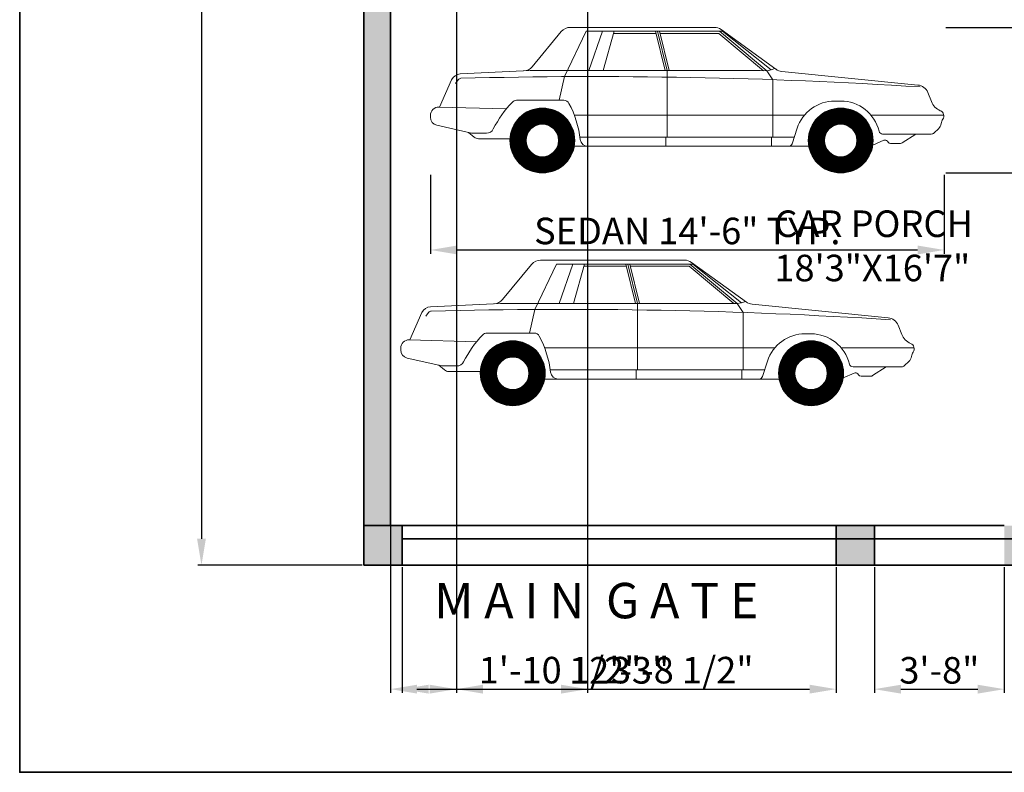
# Model space of a CAD drawing. Units: inches. Extents: x 32476 to 33108, y 58720 to 59630.
# Tile 1 of 6: x 32476 to 32810, y 58720 to 58975. Entities that reach past the tile are written whole.
import ezdxf

# ---------------------------------------------------------------- set-up
doc = ezdxf.new("R2010")
doc.units = ezdxf.units.IN
for name, color, linetype, lineweight in [('A-ANNO-DIMS', 6, 'Continuous', 18), ('A-ANNO-TEXT', 3, 'Continuous', 18), ('A-ANNO-TTLB', 7, 'Continuous', 35), ('A-AREA-IDEN', 32, 'Continuous', 18), ('A-EQPM-VEHI', 8, 'Continuous', 18), ('A-SITE-GATE', 7, 'Continuous', 35), ('A-SITE-PATT', 242, 'Continuous', 13), ('A-WALL', 7, 'Continuous', 35), ('A-WALL-PATT', 251, 'Continuous', 13)]:
    doc.layers.add(name, color=color, linetype=linetype, lineweight=lineweight)
doc.styles.get("Standard").update_dxf_attribs({"font": 'arial.ttf'})
doc.dimstyles.new('ISO-25', dxfattribs={"dimtxt": 9, "dimasz": 9, "dimexe": 1.25, "dimexo": 0.625, "dimtad": 1, "dimdec": 1, "dimrnd": 9, "dimlunit": 3, "dimtxsty": 'Standard', "dimcen": 2.5, "dimadec": 0, "dimazin": 0, "dimtfac": 1, "dimtdec": 1, "dimtmove": 0, "dimatfit": 3, "dimfxl": 1, "dimarcsym": 0})

# ---------------------------------------------------------------- blocks, each defined once
blk = doc.blocks.new('*D2')
at = {"layer": 'A-ANNO-DIMS', "color": 0, "lineweight": -2, "transparency": 16777216}
for p, q in [((32592.41, 59486.22), (32536.75, 59486.22)), ((32538, 59477.22), (32538, 58799.22)), ((32592.41, 58790.22), (32536.75, 58790.22))]:
    blk.add_line(p, q, dxfattribs=at)
at = {"layer": 'A-ANNO-DIMS', "color": 0, "transparency": 16777216}
for points in [[(32536.5, 59477.22), (32539.5, 59477.22), (32538, 59486.22)], [(32536.5, 58799.22), (32539.5, 58799.22), (32538, 58790.22)]]:
    blk.add_solid(points, dxfattribs=at)
at = {"layer": 'Defpoints', "color": 0, "transparency": 16777216}
for p in [(32593.04, 59486.22), (32538, 58790.22), (32593.04, 58790.22)]:
    blk.add_point(p, dxfattribs=at)
at = {"layer": 'A-ANNO-DIMS', "color": 0, "transparency": 16777216, "insert": (32532.78, 59138.22), "char_height": 9, "attachment_point": 5, "rotation": 90}
blk.add_mtext('57\'-9"', dxfattribs=at)
blk = doc.blocks.new('Car - sedan  side')
for p, q in [((-139.53, 35.99), (-129.64, 47.91)), ((-128.57, 32.64), (-121.22, 48.02)), ((-77.81, 49.34), (-126.58, 49.34)), ((-74.7, 48.02), (-121.22, 48.02)), ((-120.32, 34.67), (-115.67, 48.02)), ((-115.4, 34.67), (-111.74, 48.02)), ((-97.55, 47.3), (-111.94, 47.3)), ((-94.41, 34.67), (-97.73, 48.02)), ((-93.72, 34.67), (-97.04, 48.02)), ((-93.03, 34.67), (-96.34, 48.02)), ((-76.26, 47.3), (-96.16, 47.3)), ((-61.08, 34.66), (-76.26, 47.3)), ((-60.02, 34.65), (-76.07, 48.02)), ((-56.87, 35.13), (-75.48, 48.59)), ((-58.54, 34.93), (-74.99, 48.02)), ((-140.23, 34.67), (-163.88, 33.56)), ((-62.28, 34.67), (-140.23, 34.67)), ((-93.72, 19.62), (-93.72, 34.67)), ((-62.28, 34.67), (-60.02, 34.65)), ((-60.02, 34.65), (-58.54, 34.93)), ((-57.97, 31.61), (-60.02, 34.65)), ((-57.21, 35.38), (-58.54, 34.93)), ((-54.93, 34.4), (-8.75, 29.8)), ((-170.93, 22.32), (-166.81, 31.56)), ((-164.57, 31.6), (-165.48, 30.35)), ((-130.39, 24.63), (-128.57, 32.64)), ((-57.97, 19.62), (-57.97, 31.61)), ((-4.21, 24.18), (-5.42, 27.27)), ((-128.78, 24.63), (-144.79, 24.63)), ((-36.97, 24.38), (-34.94, 24.38)), ((-148.26, 21.7), (-171.11, 22.33)), ((-174, 19.51), (-174, 18.91)), ((-47.2, 19.62), (-125.23, 19.62)), ((-93.72, 12.14), (-93.72, 19.62)), ((-57.97, 12.14), (-57.97, 19.62)), ((0, 19.62), (-24.7, 19.62)), ((-160.12, 13.48), (-171.81, 16.16)), ((-159.22, 12.14), (-161.08, 13.7)), ((-155.01, 13.48), (-160.12, 13.48)), ((-51.4, 9.89), (-49.69, 15.14)), ((-3.22, 13.59), (-1.77, 14.97)), ((-147.03, 11.6), (-157.73, 11.6)), ((-50.67, 12.14), (-123.32, 12.14)), ((-94.21, 9.03), (-94.21, 12.14)), ((-58.39, 9.03), (-58.39, 12.14)), ((-20.36, 11.06), (-24.06, 9.44)), ((-4.23, 13.19), (-20.72, 13.19)), ((-18.83, 10.42), (-19.11, 10.76)), ((-14.68, 10.03), (-18.01, 10.03)), ((-9.5, 13.19), (-14.1, 10.2)), ((-120.62, 9.03), (-125.23, 9.03)), ((-45.76, 9.03), (-120.62, 9.03))]:
    blk.add_line(p, q)
at = {"const_width": 5.49}
for points in [[(-127.8, 11, -1), (-144.3, 11, -1)], [(-26.69, 11, -1), (-43.19, 11, -1)]]:
    blk.add_lwpolyline(points, format="xyb", close=True, dxfattribs=at)
for centre, radius in [((-136.05, 11), 11), ((-34.94, 11), 11), ((-136.05, 11), 5.51), ((-34.94, 11), 5.51)]:
    blk.add_circle(centre, radius)
for centre, radius, start, end in [((-126.58, 45.38), 3.97, 90, 140.3029), ((-77.81, 45.38), 3.97, 54.135, 90), ((-163.72, 30.18), 3.38, 92.6827, 155.9736), ((-142.58, 38.53), 3.97, 272.6827, 320.3029), ((-54.54, 38.35), 3.97, 234.135, 264.3123), ((-163.62, 30.91), 1.17, 91.491, 143.9553), ((-118.51, -1702.12), 1734.79, 86.34698, 91.49105), ((-9.15, 25.82), 4, 21.3107, 84.3123), ((-118.09, -2.78), 38.85, 136.3964, 152.9097), ((-144.79, 22.64), 1.98, 90, 136.3964), ((-128.78, 22.64), 1.98, 28.1371, 90), ((-157.14, 7.48), 34.14, 6.5135, 28.1371), ((-36.97, 11), 13.38, 90, 161.9732), ((-34.94, 11), 13.38, 13.5864, 90), ((0.9, 26.18), 5.49, 201.3107, 247.7048), ((-171.18, 19.51), 2.82, 88.4193, 180), ((-1.92, 19.3), 1.94, 325.3744, 67.7048), ((-171.18, 18.91), 2.82, 180, 257.0905), ((-3.82, 17.12), 2.96, 313.7173, 352.3839), ((2.46, 16.28), 3.37, 145.3744, 172.3839), ((-155.01, 16.1), 2.62, 270, 332.9097), ((-20.72, 14.43), 1.24, 193.5864, 270), ((-4.23, 14.65), 1.46, 270, 313.7173), ((-157.73, 13.93), 2.32, 230.1291, 270), ((-120.62, 11.65), 2.62, 186.5135, 270), ((-19.93, 10.09), 1.06, 39.301, 113.7159), ((-18.01, 11.09), 1.06, 219.301, 270), ((-14.68, 11.09), 1.06, 270, 303.047), ((-52.58, 10.27), 1.24, 270, 341.9732)]:
    blk.add_arc(centre, radius, start, end)
blk = doc.blocks.new('*D23')
at = {"layer": 'A-ANNO-DIMS', "color": 0, "lineweight": -2, "transparency": 16777216}
for p, q in [((32615.59, 58922.56), (32615.59, 58895.82)), ((32789.71, 58922.56), (32789.71, 58895.82)), ((32624.59, 58897.07), (32780.71, 58897.07))]:
    blk.add_line(p, q, dxfattribs=at)
at = {"layer": 'A-ANNO-DIMS', "color": 0, "transparency": 16777216}
for points in [[(32624.59, 58898.57), (32624.59, 58895.57), (32615.59, 58897.07)], [(32780.71, 58898.57), (32780.71, 58895.57), (32789.71, 58897.07)]]:
    blk.add_solid(points, dxfattribs=at)
at = {"layer": 'Defpoints', "color": 0, "transparency": 16777216}
for p in [(32615.59, 58923.18), (32789.71, 58923.18), (32789.71, 58897.07)]:
    blk.add_point(p, dxfattribs=at)
at = {"layer": 'A-ANNO-DIMS', "color": 0, "transparency": 16777216, "insert": (32702.65, 58902.35), "char_height": 9, "attachment_point": 5}
blk.add_mtext('SEDAN 14\'-6" TYP.', dxfattribs=at)
blk = doc.blocks.new('*D24')
at = {"layer": 'A-ANNO-DIMS', "color": 0, "lineweight": -2, "transparency": 16777216}
for p, q in [((32815.82, 58972.53), (32815.82, 59058.97)), ((32790.33, 58972.53), (32817.07, 58972.53)), ((32815.82, 58932.18), (32815.82, 58963.53)), ((32790.33, 58923.18), (32817.07, 58923.18))]:
    blk.add_line(p, q, dxfattribs=at)
at = {"layer": 'A-ANNO-DIMS', "color": 0, "transparency": 16777216}
for points in [[(32814.32, 58963.53), (32817.32, 58963.53), (32815.82, 58972.53)], [(32814.32, 58932.18), (32817.32, 58932.18), (32815.82, 58923.18)]]:
    blk.add_solid(points, dxfattribs=at)
at = {"layer": 'Defpoints', "color": 0, "transparency": 16777216}
for p in [(32789.71, 58972.53), (32815.82, 58972.53), (32789.71, 58923.18)]:
    blk.add_point(p, dxfattribs=at)
at = {"layer": 'A-ANNO-DIMS', "color": 0, "transparency": 16777216, "insert": (32810.54, 59020.25), "char_height": 9, "attachment_point": 5, "rotation": 90}
blk.add_mtext('4\'-1 1/2" TYP.', dxfattribs=at)
blk = doc.blocks.new('*D37')
at = {"layer": 'A-ANNO-DIMS', "color": 0, "lineweight": -2, "transparency": 16777216}
for p, q in [((32605.97, 58789.59), (32605.97, 58746.97)), ((32753.12, 58789.59), (32753.12, 58746.97)), ((32614.97, 58748.22), (32744.12, 58748.22))]:
    blk.add_line(p, q, dxfattribs=at)
at = {"layer": 'A-ANNO-DIMS', "color": 0, "transparency": 16777216}
for points in [[(32614.97, 58749.72), (32614.97, 58746.72), (32605.97, 58748.22)], [(32744.12, 58749.72), (32744.12, 58746.72), (32753.12, 58748.22)]]:
    blk.add_solid(points, dxfattribs=at)
at = {"layer": 'Defpoints', "color": 0, "transparency": 16777216}
for p in [(32605.97, 58790.22), (32753.12, 58790.22), (32753.12, 58748.22)]:
    blk.add_point(p, dxfattribs=at)
at = {"layer": 'A-ANNO-DIMS', "color": 0, "transparency": 16777216, "insert": (32679.55, 58753.44), "char_height": 9, "attachment_point": 5}
blk.add_mtext('12\'-3"', dxfattribs=at)
blk = doc.blocks.new('*D38')
at = {"layer": 'A-ANNO-DIMS', "color": 0, "lineweight": -2, "transparency": 16777216}
for p, q in [((32766.06, 58789.59), (32766.06, 58746.97)), ((32810.1, 58789.59), (32810.1, 58746.97)), ((32775.06, 58748.22), (32801.1, 58748.22))]:
    blk.add_line(p, q, dxfattribs=at)
at = {"layer": 'A-ANNO-DIMS', "color": 0, "transparency": 16777216}
for points in [[(32775.06, 58749.72), (32775.06, 58746.72), (32766.06, 58748.22)], [(32801.1, 58749.72), (32801.1, 58746.72), (32810.1, 58748.22)]]:
    blk.add_solid(points, dxfattribs=at)
at = {"layer": 'Defpoints', "color": 0, "transparency": 16777216}
for p in [(32766.06, 58790.22), (32810.1, 58790.22), (32810.1, 58748.22)]:
    blk.add_point(p, dxfattribs=at)
at = {"layer": 'A-ANNO-DIMS', "color": 0, "transparency": 16777216, "insert": (32788.08, 58753.44), "char_height": 9, "attachment_point": 5}
blk.add_mtext('3\'-8"', dxfattribs=at)
blk = doc.blocks.new('*D45')
at = {"layer": 'A-ANNO-DIMS', "color": 0, "lineweight": -2, "transparency": 16777216}
for p, q in [((32602.04, 59010.09), (32602.04, 58746.97)), ((32624.39, 59010.09), (32624.39, 58746.97)), ((32611.04, 58748.22), (32615.39, 58748.22)), ((32624.39, 58748.22), (32685.68, 58748.22))]:
    blk.add_line(p, q, dxfattribs=at)
at = {"layer": 'A-ANNO-DIMS', "color": 0, "transparency": 16777216}
for points in [[(32611.04, 58749.72), (32611.04, 58746.72), (32602.04, 58748.22)], [(32615.39, 58749.72), (32615.39, 58746.72), (32624.39, 58748.22)]]:
    blk.add_solid(points, dxfattribs=at)
at = {"layer": 'Defpoints', "color": 0, "transparency": 16777216}
for p in [(32602.04, 59010.72), (32624.39, 59010.72), (32624.39, 58748.22)]:
    blk.add_point(p, dxfattribs=at)
at = {"layer": 'A-ANNO-DIMS', "color": 0, "transparency": 16777216, "insert": (32659.53, 58753.5), "char_height": 9, "attachment_point": 5}
blk.add_mtext('1\'-10 1/2"', dxfattribs=at)
blk = doc.blocks.new('*D46')
at = {"layer": 'A-ANNO-DIMS', "color": 0, "lineweight": -2, "transparency": 16777216}
for p, q in [((32624.39, 59010.09), (32624.39, 58746.97)), ((32668.87, 59010.09), (32668.87, 58746.97)), ((32633.39, 58748.22), (32659.87, 58748.22)), ((32668.87, 58748.22), (32724.01, 58748.22))]:
    blk.add_line(p, q, dxfattribs=at)
at = {"layer": 'A-ANNO-DIMS', "color": 0, "transparency": 16777216}
for points in [[(32633.39, 58749.72), (32633.39, 58746.72), (32624.39, 58748.22)], [(32659.87, 58749.72), (32659.87, 58746.72), (32668.87, 58748.22)]]:
    blk.add_solid(points, dxfattribs=at)
at = {"layer": 'Defpoints', "color": 0, "transparency": 16777216}
for p in [(32624.39, 59010.72), (32668.87, 59010.72), (32668.87, 58748.22)]:
    blk.add_point(p, dxfattribs=at)
at = {"layer": 'A-ANNO-DIMS', "color": 0, "transparency": 16777216, "insert": (32700.94, 58753.5), "char_height": 9, "attachment_point": 5}
blk.add_mtext('3\'-8 1/2"', dxfattribs=at)

msp = doc.modelspace()

# ---------------------------------------------------------------- hatches: boundary and pattern name
at = {"layer": 'A-SITE-PATT'}
h = msp.add_hatch(color=256, dxfattribs=at)
h.dxf.hatch_style = 1
h.paths.add_polyline_path([(32605.97, 58803.66), (32593.04, 58803.66), (32593.04, 58790.22), (32605.97, 58790.22)])
h.paths.add_polyline_path([(32766.06, 58799.22), (32753.12, 58799.22), (32753.12, 58790.22), (32766.06, 58790.22)])
h.paths.add_polyline_path([(32766.06, 58803.66), (32753.12, 58803.66), (32753.12, 58799.22), (32766.06, 58799.22)])
h.paths.add_polyline_path([(32823.04, 58799.22), (32810.1, 58799.22), (32810.1, 58790.22), (32823.04, 58790.22)])
h.paths.add_polyline_path([(32823.04, 58803.66), (32810.1, 58803.66), (32810.1, 58799.22), (32823.04, 58799.22)])
at = {"layer": 'A-WALL-PATT'}
h = msp.add_hatch(color=256, dxfattribs=at)
h.dxf.hatch_style = 1
h.paths.add_polyline_path([(32602.04, 59418.72), (32606.39, 59418.72), (32606.39, 59423.22), (32602.04, 59423.22), (32602.04, 59477.22), (32698.04, 59477.22), (32698.04, 59469.73), (32702.54, 59469.73), (32702.54, 59481.72), (32867.54, 59481.72), (32867.54, 59427.72), (32860.2, 59427.72), (32860.2, 59418.72), (32867.54, 59418.72), (32935.14, 59418.72), (32935.14, 59423.22), (32872.04, 59423.22), (32872.04, 59477.22), (32968.04, 59477.22), (32968.04, 59423.22), (32962.36, 59423.22), (32962.36, 59418.72), (32968.04, 59418.72), (32968.04, 59286.72), (32867.54, 59286.72), (32832.04, 59286.72), (32828.7, 59289.44), (32818.99, 59279.82), (32823.04, 59277.72), (32823.04, 59269.52), (32832.04, 59269.52), (32832.04, 59277.72), (32867.54, 59277.72), (32968.04, 59277.72), (32968.04, 58880.22), (32925.88, 58880.22), (32925.88, 58871.22), (32968.04, 58871.22), (32968.04, 58799.22), (32823.04, 58799.22), (32823.04, 58790.22), (32977.04, 58790.22), (32977.04, 59486.22), (32867.54, 59486.22), (32702.54, 59486.22), (32593.04, 59486.22), (32593.04, 58803.66), (32602.04, 58803.66), (32602.04, 59001.72), (32624.39, 59001.72), (32624.39, 59010.72), (32602.04, 59010.72), (32602.04, 59124.72), (32648.65, 59124.72), (32648.65, 59133.72), (32602.04, 59133.72), (32602.04, 59277.72), (32757.41, 59277.72), (32757.41, 59279.22), (32742.07, 59288.84), (32739.6, 59286.72), (32702.54, 59286.72), (32602.04, 59286.72)])
h.paths.add_polyline_path([(32763.92, 59133.72), (32685.69, 59133.72), (32685.69, 59124.72), (32693.04, 59124.72), (32693.04, 59010.72), (32668.87, 59010.72), (32668.87, 59001.72), (32705.76, 59001.72), (32705.76, 59010.72), (32702.04, 59010.72), (32702.04, 59124.72), (32763.92, 59124.72)], flags=17)
h.paths.add_polyline_path([(32832.04, 59226.49), (32823.04, 59226.49), (32823.04, 59133.72), (32814.31, 59133.72), (32814.31, 59124.72), (32823.04, 59124.72), (32823.04, 59099.14), (32832.04, 59099.14), (32832.04, 59124.72), (32839.29, 59124.72), (32839.29, 59133.72), (32832.04, 59133.72)], flags=17)
h.paths.add_polyline_path([(32921.54, 59133.72), (32874.43, 59133.72), (32874.43, 59124.72), (32917.04, 59124.72), (32917.04, 59097.72), (32921.54, 59097.72), (32921.54, 59124.72)], flags=17)
h.paths.add_polyline_path([(32832.04, 59066.22), (32968.04, 59066.22), (32968.04, 59070.72), (32921.54, 59070.72), (32921.54, 59074.56), (32917.04, 59074.56), (32917.04, 59070.72), (32832.04, 59070.72), (32832.04, 59074.32), (32823.04, 59074.32), (32823.04, 59056.98), (32832.04, 59056.98)], flags=17)
h.paths.add_polyline_path([(32738.1, 59010.72), (32721.79, 59010.72), (32721.79, 59001.72), (32738.1, 59001.72)], flags=16)
h.paths.add_polyline_path([(32763.19, 59010.72), (32754.77, 59010.72), (32754.77, 59001.72), (32763.19, 59001.72)], flags=16)
h.paths.add_polyline_path([(32832.04, 59016.15), (32823.04, 59016.15), (32823.04, 59010.72), (32814.31, 59010.72), (32814.31, 59001.72), (32823.04, 59001.72), (32823.04, 58871.22), (32860.05, 58871.22), (32860.05, 58880.22), (32832.04, 58880.22)], flags=17)
h.paths.add_polyline_path([(32702.54, 59448.33), (32698.04, 59448.33), (32698.04, 59423.22), (32631.9, 59423.22), (32631.9, 59418.72), (32702.54, 59418.72), (32706.18, 59418.72), (32706.18, 59427.72), (32702.54, 59427.72)], flags=17)
h.paths.add_polyline_path([(32789.04, 59418.72), (32800.22, 59418.72), (32800.22, 59427.72), (32775.59, 59427.72), (32775.59, 59418.72), (32780.04, 59418.72), (32780.04, 59337.58), (32773.73, 59333.67), (32782.91, 59322.03), (32784.1, 59324.11), (32785.3, 59322.03), (32798.33, 59329.69), (32789.04, 59343.18)], flags=17)

# ---------------------------------------------------------------- linework, layer by layer
at = {"layer": 'A-ANNO-TTLB'}
msp.add_lwpolyline([(32476.39, 59629.64), (33046.1, 59629.64), (33046.1, 58720.03), (32476.39, 58720.03)], close=True, dxfattribs=at)
at = {"layer": 'A-SITE-GATE'}
for p, q in [((32605.97, 58803.66), (32753.12, 58803.66)), ((32766.06, 58803.66), (32810.1, 58803.66))]:
    msp.add_line(p, q, dxfattribs=at)
for points in [[(32593.04, 58790.22), (32605.97, 58790.22), (32605.97, 58803.66), (32593.04, 58803.66)], [(32753.12, 58790.22), (32766.06, 58790.22), (32766.06, 58803.66), (32753.12, 58803.66)]]:
    msp.add_lwpolyline(points, close=True, dxfattribs=at)
at = {"layer": 'A-WALL'}
for p, q in [((32593.04, 59486.22), (32593.04, 58790.22)), ((32602.04, 59001.72), (32602.04, 58803.66)), ((32605.97, 58799.22), (32968.04, 58799.22)), ((32593.04, 58790.22), (32977.04, 58790.22))]:
    msp.add_line(p, q, dxfattribs=at)

# ---------------------------------------------------------------- block references
at = {"layer": 'A-EQPM-VEHI'}
for p in [(32789.59, 58923.18), (32779.54, 58844.28)]:
    msp.add_blockref('Car - sedan  side', p, dxfattribs=at)

# ---------------------------------------------------------------- texts
at = {"layer": 'A-ANNO-TEXT', "insert": (32616.88, 58784.24), "char_height": 12, "attachment_point": 1}
msp.add_mtext_dynamic_manual_height_columns('M A I N  G A T E', width=127.6543, gutter_width=12.5, heights=[0], dxfattribs=at)
at = {"layer": 'A-AREA-IDEN', "insert": (32732.16, 58910.47), "char_height": 9, "attachment_point": 1}
msp.add_mtext_dynamic_manual_height_columns('CAR PORCH\\P18\'3"X16\'7"', width=113.927, gutter_width=12.5, heights=[0], dxfattribs=at)

# ---------------------------------------------------------------- dimensions: what is measured, and where the dimension line sits
at = {"layer": 'A-ANNO-DIMS'}
dim = msp.add_linear_dim(base=(32538, 58790.22), p1=(32593.04, 59486.22), p2=(32593.04, 58790.22), angle=90, dimstyle='ISO-25', override={"dimclrd": 0, "dimclre": 0, "dimclrt": 0}, dxfattribs=at)
dim.commit()
dim.dimension.update_dxf_attribs({"geometry": '*D2', "text_midpoint": (32532.78, 59138.22)})
dim = msp.add_linear_dim(base=(32815.8223, 58972.5292), p1=(32789.7053, 58923.1843), p2=(32789.7053, 58972.5292), angle=90, text='<> TYP.', dimstyle='ISO-25', override={"dimdec": 1, "dimlfac": 1, "dimrnd": 0, "dimzin": 1, "dimdsep": 46, "dimlunit": 4, "dimfrac": 2}, dxfattribs=at)
dim.commit()
dim.dimension.update_dxf_attribs({"geometry": '*D24', "text_midpoint": (32810.5439, 59020.2507)})
for base, p1, p2, picture, middle in [((32624.3879, 58748.2191), (32602.0354, 59010.7191), (32624.3879, 59010.7191), '*D45', (32659.5334, 58753.4976)), ((32668.87, 58748.22), (32624.39, 59010.72), (32668.87, 59010.72), '*D46', (32700.94, 58753.5)), ((32753.1237, 58748.2191), (32605.9707, 58790.2191), (32753.1237, 58790.2191), '*D37', (32679.5472, 58753.4423)), ((32810.1, 58748.22), (32766.06, 58790.22), (32810.1, 58790.22), '*D38', (32788.08, 58753.44))]:
    dim = msp.add_linear_dim(base=base, p1=p1, p2=p2, dimstyle='ISO-25', override={"dimdec": 1, "dimlfac": 1, "dimrnd": 0, "dimzin": 1, "dimdsep": 46, "dimlunit": 4, "dimfrac": 2}, dxfattribs=at)
    dim.commit()
    dim.dimension.update_dxf_attribs({"geometry": picture, "text_midpoint": middle})
dim = msp.add_linear_dim(base=(32789.71, 58897.07), p1=(32615.59, 58923.18), p2=(32789.71, 58923.18), text='SEDAN <> TYP.', dimstyle='ISO-25', override={"dimdec": 1, "dimlfac": 1, "dimrnd": 0, "dimzin": 1, "dimdsep": 46, "dimlunit": 4, "dimfrac": 2}, dxfattribs=at)
dim.commit()
dim.dimension.update_dxf_attribs({"geometry": '*D23', "text_midpoint": (32702.65, 58902.35)})

doc.saveas('drawing.dxf')
